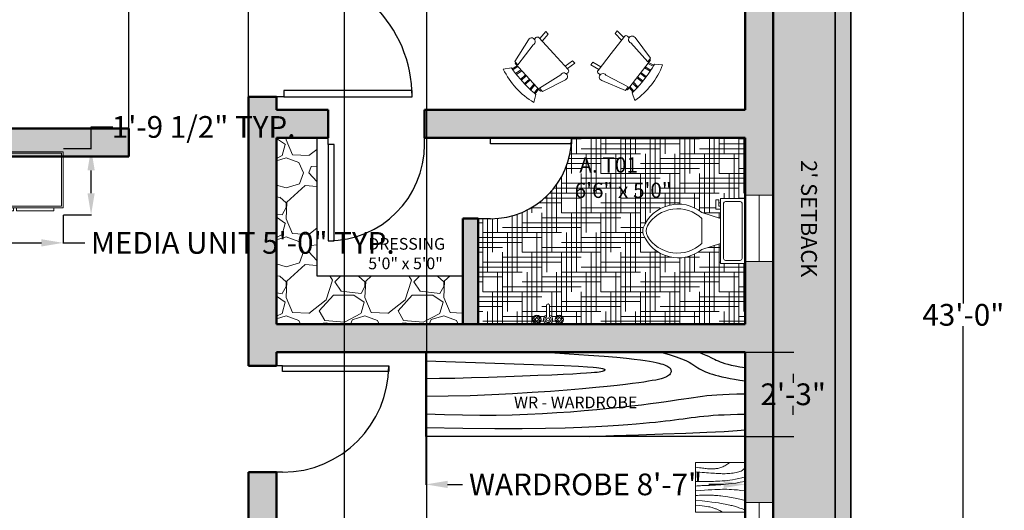
# Model space of a CAD drawing. Units: inches. Extents: x 319 to 870, y 210 to 995.
# Tile 5 of 6: x 524 to 841, y 603 to 761. Entities that reach past the tile are written whole.
import ezdxf

# ---------------------------------------------------------------- set-up
doc = ezdxf.new("R2010")
doc.units = ezdxf.units.IN
doc.header["$MEASUREMENT"] = 0
for name, color, linetype, lineweight in [('A-ANNO-DIMS', 2, 'Continuous', 18), ('A-ANNO-TEXT', 7, 'Continuous', 18), ('A-AREA-IDEN', 7, 'Continuous', 18), ('A-DOOR', 4, 'Continuous', 25), ('A-FLOR-CASE', 7, 'Continuous', 25), ('A-FLOR-CASE-PATT', 252, 'Continuous', 13), ('A-FLOR-FIXT', 9, 'Continuous', 18), ('A-FLOR-PATT', 252, 'Continuous', 13), ('A-FURN', 8, 'Continuous', 18), ('A-GLAZ', 4, 'Continuous', 18), ('A-WALL', 7, 'Continuous', 50), ('A-WALL-PATT', 8, 'Continuous', 13), ('C-PROP', 7, 'Continuous', 35), ('C-PROP-PATT', 8, 'Continuous', 13)]:
    doc.layers.add(name, color=color, linetype=linetype, lineweight=lineweight)
doc.layers.add('C-SITE-PATT', color=126, linetype='Continuous', lineweight=13, true_color=0x1e6f63)
doc.styles.get("Standard").update_dxf_attribs({"font": 'arial.ttf'})
doc.dimstyles.get("Standard").update_dxf_attribs({"dimtxt": 7, "dimasz": 7, "dimexe": 0.18, "dimexo": 0.0625, "dimgap": 0.09, "dimtad": 0, "dimtih": 1, "dimtoh": 1, "dimdec": 0, "dimzin": 0, "dimdsep": 46, "dimlunit": 3, "dimtxsty": 'Standard', "dimcen": 0.09, "dimadec": 0, "dimazin": 0, "dimtfac": 1, "dimtdec": 0, "dimtofl": 0, "dimtmove": 0, "dimatfit": 3, "dimfxl": 1, "dimtolj": 1, "dimtzin": 0, "dimarcsym": 0})

# ---------------------------------------------------------------- blocks, each defined once
blk = doc.blocks.new('Toilet - top')
for p, q in [((9.5, -6), (9.5, -2)), ((-10, -8.5), (-8, -8.5)), ((-10, -9.5), (-10, -8.5)), ((-7, -9.5), (-10, -9.5)), ((-8, -8.5), (-8, -8)), ((-7, -8), (-7, -9.5)), ((-4, -8), (-6, -14)), ((4, -8), (6, -14)), ((4, -14), (-4, -14))]:
    blk.add_line(p, q)
blk.add_lwpolyline([(10.5, -8), (10.5, 0), (-10.5, 0), (-10.5, -8)], close=True)
for points in [[(-9.5, -2), (-9.5, -6)], [(8.5, -1), (-8.5, -1)], [(-8.5, -7), (8.5, -7)]]:
    blk.add_lwpolyline(points)
for centre, radius, start, end in [((-8.62, -1.88), 0.884, 81.8699, 188.1301), ((8.62, -1.88), 0.884, 351.8699, 98.1301), ((-8.62, -6.12), 0.884, 171.8699, 278.1301), ((8.62, -6.12), 0.884, 261.8699, 8.1301), ((3.52, -21.58), 12.17, 141.4691, 247.9714), ((4.2, -21.82), 11.33, 136.3677, 238.9468), ((-3.52, -21.58), 12.17, 292.0284, 38.5307), ((-4.2, -21.82), 11.33, 301.053, 43.6321), ((0, -27.88), 4, 245.7318, 294.2682), ((0, -29), 4, 254.8605, 285.1395)]:
    blk.add_arc(centre, radius, start, end)
blk = doc.blocks.new('Faucet - Bathroom top')
for p, q in [((-4.107, 0.125), (-4.375, 0.125)), ((-3.75, 0.4788), (-3.75, 0.75)), ((-3.5, 0.482), (-3.5, 0.75)), ((-3.1461, 0.125), (-2.875, 0.125)), ((3.143, 0.125), (2.875, 0.125)), ((3.5, 0.4788), (3.5, 0.75)), ((3.75, 0.482), (3.75, 0.75)), ((4.1039, 0.125), (4.375, 0.125)), ((-4.1039, -0.125), (-4.375, -0.125)), ((-3.75, -0.4821), (-3.75, -0.75)), ((-3.5, -0.4789), (-3.5, -0.75)), ((-3.143, -0.125), (-2.875, -0.125)), ((-0.5, -0.8639), (-0.5, -4.5)), ((0.5, -4.5), (0.5, -0.8631)), ((3.1461, -0.125), (2.875, -0.125)), ((3.5, -0.4821), (3.5, -0.75)), ((3.75, -0.4789), (3.75, -0.75)), ((4.107, -0.125), (4.375, -0.125))]:
    blk.add_line(p, q)
for centre, radius in [((-3.625, 0), 1.375), ((-4.625, 0), 0.2795), ((-3.625, 0), 0.5), ((-3.625, 1), 0.2795), ((-2.625, 0), 0.2795), ((0, 0), 0.5), ((3.625, 0), 1.375), ((2.625, 0), 0.2795), ((3.625, 0), 0.5), ((3.625, 1), 0.2795), ((4.625, 0), 0.2795), ((-3.625, -1), 0.2795), ((3.625, -1), 0.2795)]:
    blk.add_circle(centre, radius)
for centre, radius, start, end in [((-3.625, 0), 1, 105.2407, 164.2093), ((-3.625, 0), 1, 16.44125, 74.07887), ((0, 0), 1.5, 289.6514, 250.3603), ((0, 0), 1, 300.3431, 239.7554), ((3.625, 0), 1, 106.12, 164.0884), ((3.625, 0), 1, 16.23422, 73.90469), ((-3.625, 0), 1, 196.2342, 253.9047), ((-3.625, 0), 1, 286.12, 344.0884), ((3.625, 0), 1, 196.4413, 254.0789), ((3.625, 0), 1, 285.2407, 344.2093), ((0, -4.5), 0.5, 180, 0)]:
    blk.add_arc(centre, radius, start, end)
blk = doc.blocks.new('*U14')
for p, q in [((0, 0), (0, -6)), ((-36, 0), (-36, -6))]:
    blk.add_line(p, q)
blk.add_lwpolyline([(0, 0), (0, 36), (-1.75, 36), (-1.75, 0)], close=True)
blk.add_arc((0, 0), 36, 90, 180)
blk = doc.blocks.new('*U15')
for p, q in [((-28, 0), (-28, -6)), ((0, 0), (0, -6))]:
    blk.add_line(p, q)
blk.add_lwpolyline([(0, 0), (0, 28), (-1.75, 28), (-1.75, 0)], close=True)
blk.add_arc((0, 0), 28, 90, 180)
blk = doc.blocks.new('*U16')
for p, q in [((0, 0), (0, -6)), ((32, 0), (32, -6))]:
    blk.add_line(p, q)
blk.add_lwpolyline([(0, 0), (0, 32), (1.75, 32), (1.75, 0)], close=True)
blk.add_arc((0, 0), 32, 0, 90)
blk = doc.blocks.new('Hutch - 19 x 72 in.')
for p, q in [((0, -19), (0, 0)), ((0, 0), (71.999994, 0)), ((71.999994, 0), (71.999994, -19)), ((71.999994, -19), (0, -19))]:
    blk.add_line(p, q)
for points in [[(26.99999, 0), (32.30411, -0.35238), (36.66731, -0.66276), (40.20336, -0.93603), (43.02603, -1.17708), (45.2491, -1.39079), (46.98632, -1.58203), (48.35147, -1.7557), (49.45833, -1.91667), (50.40388, -2.06917), (51.21809, -2.21484), (51.91414, -2.35465), (52.5052, -2.48958), (53.00447, -2.6206), (53.42512, -2.7487), (53.78035, -2.87484), (54.08333, -3), (54.34537, -3.12516), (54.57031, -3.2513), (54.76008, -3.37939), (54.91666, -3.51042), (55.04198, -3.64534), (55.13801, -3.78516), (55.2067, -3.93083), (55.24999, -4.08333), (55.26904, -4.24316), (55.26171, -4.40885), (55.22509, -4.57845), (55.15624, -4.75), (55.05224, -4.92155), (54.91015, -5.09115), (54.72704, -5.25684), (54.49999, -5.41667), (54.22493, -5.56934), (53.89322, -5.71615), (53.49511, -5.85905), (53.02083, -6), (52.4606, -6.14095), (51.80468, -6.28385), (51.04329, -6.43066), (50.16666, -6.58333), (49.16007, -6.74381), (47.98892, -6.91406), (46.61368, -7.09603), (44.99478, -7.29167), (43.09268, -7.50293), (40.86783, -7.73177), (38.28067, -7.98014), (35.29166, -8.25), (31.87654, -8.54053), (28.07226, -8.83984), (23.93107, -9.1333), (19.5052, -9.40625), (14.84692, -9.64404), (10.00846, -9.83203), (5.04207, -9.95557), (0, -10)], [(52.99999, 0), (54.87133, -0.53955), (56.39257, -1.03516), (57.61205, -1.48975), (58.57812, -1.90625), (59.3391, -2.2876), (59.94335, -2.63672), (60.4392, -2.95654), (60.87499, -3.25), (61.29247, -3.52002), (61.70702, -3.76953), (62.12743, -4.00146), (62.56249, -4.21875), (63.02099, -4.42432), (63.51171, -4.62109), (64.04345, -4.81201), (64.62499, -5), (65.26489, -5.1875), (65.9707, -5.375), (66.74975, -5.5625), (67.60937, -5.75), (68.55688, -5.9375), (69.5996, -6.125), (70.744867, -6.3125), (71.999994, -6.5)], [(61.49999, 0), (62.35961, -0.35254), (63.08007, -0.66406), (63.68627, -0.94043), (64.20312, -1.1875), (64.65551, -1.41113), (65.06835, -1.61719), (65.46655, -1.81152), (65.87499, -2), (66.31762, -2.1875), (66.81445, -2.375), (67.38452, -2.5625), (68.04687, -2.75), (68.82055, -2.9375), (69.7246, -3.125), (70.77807, -3.3125), (71.999994, -3.5)], [(0, -2), (11.2006, -2.34123), (19.90169, -2.62044), (26.43969, -2.84595), (31.15103, -3.02604), (34.37214, -3.16903), (36.43945, -3.2832), (37.68936, -3.37687), (38.45833, -3.45833), (39.02937, -3.53459), (39.472, -3.60742), (39.80232, -3.67733), (40.03645, -3.74479), (40.1905, -3.8103), (40.28059, -3.87435), (40.32283, -3.93742), (40.33333, -4), (40.32405, -4.0625), (40.29036, -4.125), (40.22346, -4.1875), (40.11458, -4.25), (39.95491, -4.3125), (39.73567, -4.375), (39.44807, -4.4375), (39.08333, -4.5), (38.62491, -4.56282), (38.02538, -4.6276), (37.22957, -4.69629), (36.18228, -4.77083), (34.82836, -4.85319), (33.11262, -4.94531), (30.97989, -5.04915), (28.37499, -5.16667), (25.27416, -5.29818), (21.77929, -5.4375), (18.02368, -5.57682), (14.14062, -5.70833), (10.26342, -5.82422), (6.52539, -5.91667), (3.05981, -5.97786), (0, -6)], [(71.999994, -9.5), (70.071934, -9.51147), (68.38801, -9.54492), (66.91113, -9.59888), (65.60416, -9.67187), (64.43001, -9.76245), (63.35156, -9.86914), (62.3317, -9.99048), (61.33333, -10.125), (60.32128, -10.27157), (59.26822, -10.43034), (58.14876, -10.60181), (56.93749, -10.78646), (55.60904, -10.98478), (54.13801, -11.19726), (52.49902, -11.4244), (50.66666, -11.66667), (48.62239, -11.92358), (46.37499, -12.19075), (43.9401, -12.46281), (41.33333, -12.73437), (38.57031, -13.00008), (35.66666, -13.25456), (32.63801, -13.49243), (29.49999, -13.70833), (26.26367, -13.89689), (22.92187, -14.05273), (19.46289, -14.17049), (15.875, -14.24479), (12.14648, -14.27026), (8.26562, -14.24154), (4.2207, -14.15324), (0, -14)], [(0, -17), (8.37556, -17.14274), (15.58268, -17.20443), (21.74194, -17.19775), (26.97395, -17.13542), (31.39933, -17.03011), (35.13866, -16.89453), (38.31257, -16.74137), (41.04166, -16.58333), (43.4322, -16.43083), (45.5332, -16.28516), (47.37931, -16.14534), (49.0052, -16.01042), (50.44555, -15.87939), (51.73502, -15.7513), (52.90828, -15.62516), (53.99999, -15.5), (55.04044, -15.37508), (56.04231, -15.25065), (57.01391, -15.1272), (57.96353, -15.00521), (58.89949, -14.88517), (59.83007, -14.76758), (60.76358, -14.65291), (61.70833, -14.54167), (62.6752, -14.43465), (63.68554, -14.33398), (64.76326, -14.24211), (65.93229, -14.16146), (67.21655, -14.09448), (68.63997, -14.04362), (70.226475, -14.01131), (71.999994, -14)], [(36.99999, -19), (42.40038, -18.8125), (47.95312, -18.625), (53.43554, -18.4375), (58.62499, -18.25), (63.29882, -18.0625), (67.23437, -17.875), (70.208978, -17.6875), (71.999994, -17.5)]]:
    blk.add_lwpolyline(points)
blk = doc.blocks.new('Entertainment Center')
for p, q in [((-4, 0), (-5, -1)), ((4, 0), (-4, 0)), ((5, -1), (4, 0)), ((-17, -19), (-17, -1)), ((-17, -1), (43, -1)), ((-16.5, -18.5), (-16.5, -1.5)), ((-16.5, -1.5), (42.5, -1.5)), ((42.5, -1.5), (42.5, -18.5)), ((43, -1), (43, -19)), ((43, -19), (-17, -19)), ((42.5, -18.5), (-16.5, -18.5)), ((-12, -20), (-12, -19)), ((12, -19), (12, -20)), ((15, -20), (15, -19)), ((27, -19), (27, -20)), ((28, -20), (28, -19)), ((40, -19), (40, -20)), ((12, -20), (-12, -20)), ((27, -20), (15, -20)), ((40, -20), (28, -20))]:
    blk.add_line(p, q)
blk.add_arc((0, 40), 61, 259.6111, 280.3889)
blk = doc.blocks.new('Chair - Rocking')
for p, q in [((-8, -4.5), (-10, -1.5)), ((-4.5, -7), (-4.96674, -4.19951)), ((-4, -7), (-4.40532, -4.16272)), ((-1.5, -4.05012), (-1.5, -7)), ((-1, -7), (-1, -4.05012)), ((1, -7), (1, -4.04655)), ((1.5, -4.05012), (1.5, -7)), ((4, -7), (4.40187, -4.18694)), ((4.5, -7), (4.96761, -4.19437)), ((8, -4.5), (10, -1.5)), ((-9, -7.5), (-12, -18.49999)), ((-7, -7.5), (-9, -7.5)), ((-9, -18.49999), (-7, -7.5)), ((-8.23428, -6.99939), (-8.3093, -7.47958)), ((-8.23041, -7), (8.23915, -7)), ((-7.5, -4.5), (-7, -7)), ((-6.5, -7), (-7.02225, -4.43)), ((6.5, -7), (7, -4.4057)), ((7.5, -4.5), (7, -7)), ((7, -7.5), (9, -7.5)), ((9, -18.49999), (7, -7.5)), ((8.31071, -7.48854), (8.23449, -7.00073)), ((9, -7.5), (12, -18.49999)), ((-10.36644, -20.64523), (-10.5, -21.49999)), ((10.5, -21.49999), (10.3575, -20.58798)), ((-9, -22.49999), (-9.5, -26.49999)), ((0, -22.49999), (-9.5, -22.49999)), ((-8, -26.49999), (-7.5, -22.49999)), ((0, -22.49999), (9.5, -22.49999)), ((8, -26.49999), (7.5, -22.49999)), ((9, -22.49999), (9.5, -26.49999)), ((-9.5, -26.49999), (-8, -26.49999)), ((9.5, -26.49999), (8, -26.49999))]:
    blk.add_line(p, q)
for centre, radius, start, end in [((0, -34.08333), 34.08333, 72.93847, 107.0615), ((0, -68.25004), 64.25, 93.92211, 97.15267), ((0, -68.25004), 64.25, 82.84733, 93.92211), ((-10.5, -18.99999), 1.58114, 161.5651, 18.43495), ((-9.5, -21.49999), 1, 180, 270), ((10.5, -18.99999), 1.58114, 161.5651, 18.43495), ((9.5, -21.49999), 1, 270, 0)]:
    blk.add_arc(centre, radius, start, end)
blk = doc.blocks.new('Table - Square Woodgrain 42 x 42 in.')
blk.add_line((0, -42), (42, -42))
for points in [[(0, -4), (1.704, -4.2172), (3.2358, -4.4188), (4.615, -4.604), (5.8615, -4.7721), (6.9951, -4.9224), (8.0357, -5.0541), (9.0031, -5.1667), (9.9171, -5.2594), (10.7951, -5.3316), (11.6445, -5.3836), (12.4702, -5.4157), (13.277, -5.4283), (14.0698, -5.4217), (14.8535, -5.3964), (15.6331, -5.3526), (16.4133, -5.2908), (17.1986, -5.2103), (17.9913, -5.1062), (18.793, -4.9727), (19.6056, -4.8038), (20.4307, -4.5937), (21.2701, -4.3365), (22.1256, -4.0262), (22.9989, -3.6571), (23.888, -3.2272), (24.7756, -2.7516), (25.6408, -2.2491), (26.4624, -1.7387), (27.2195, -1.2395), (27.891, -0.7703), (28.456, -0.3501), (28.8934, 0.002)], [(0, -42), (0, 0), (42, 0), (42, -42)], [(0, -8), (1.8203, -8.1001), (3.6741, -8.2149), (5.5411, -8.3408), (7.4011, -8.4741), (9.2339, -8.6112), (11.0193, -8.7484), (12.7371, -8.8821), (14.3671, -9.0086), (15.8954, -9.1246), (17.3337, -9.2278), (18.6997, -9.3159), (20.0116, -9.387), (21.2871, -9.4389), (22.5442, -9.4696), (23.8008, -9.477), (25.0749, -9.459), (26.3791, -9.4137), (27.7049, -9.3403), (29.0383, -9.2382), (30.3655, -9.1068), (31.6728, -8.9455), (32.9461, -8.7535), (34.1717, -8.5304), (35.3358, -8.2756), (36.4268, -7.9863), (37.443, -7.6521), (38.3849, -7.2603), (39.253, -6.7986), (40.048, -6.2542), (40.7705, -5.6147), (41.421, -4.8674), (42, -4)], [(42, -12), (39.1784, -12.8621), (36.4519, -13.5654), (33.8246, -14.1294), (31.3004, -14.5731), (28.8832, -14.9161), (26.577, -15.1775), (24.3858, -15.3768), (22.3136, -15.5332), (20.3622, -15.6632), (18.5254, -15.7718), (16.7947, -15.8612), (15.1618, -15.9338), (13.6183, -15.9916), (12.1558, -16.0369), (10.7659, -16.0718), (9.4403, -16.0987), (8.1703, -16.1191), (6.9461, -16.1325), (5.7577, -16.1377), (4.595, -16.1335), (3.4479, -16.1188), (2.3064, -16.0924), (1.1604, -16.0532), (0, -16)], [(42, -16), (37.6529, -16.7365), (33.8802, -17.329), (30.6179, -17.7961), (27.8015, -18.1561), (25.3668, -18.4275), (23.2497, -18.6288), (21.3859, -18.7785), (19.7111, -18.8949), (18.1693, -18.9939), (16.7375, -19.0795), (15.401, -19.1534), (14.1449, -19.217), (12.9544, -19.2717), (11.8148, -19.3191), (10.7113, -19.3606), (9.6291, -19.3976), (8.5534, -19.4323), (7.47, -19.4689), (6.3643, -19.5122), (5.222, -19.5672), (4.0288, -19.6386), (2.7703, -19.7313), (1.4321, -19.8501), (0, -20)], [(0, -24), (3.9243, -23.6805), (7.4766, -23.4138), (10.6891, -23.1954), (13.5943, -23.0205), (16.2247, -22.8847), (18.6125, -22.7832), (20.7903, -22.7116), (22.7903, -22.6651), (24.6563, -22.642), (26.4764, -22.6507), (28.35, -22.7024), (30.3766, -22.8084), (32.6555, -22.98), (35.2861, -23.2283), (38.3678, -23.5645), (42, -24)], [(42, -32), (37.392, -31.017), (33.4585, -30.2231), (30.1291, -29.5949), (27.3334, -29.109), (25.0009, -28.742), (23.0612, -28.4707), (21.4439, -28.2716), (20.0786, -28.1215), (18.8998, -28.0002), (17.8609, -27.9014), (16.9206, -27.8219), (16.0371, -27.7588), (15.1691, -27.709), (14.2748, -27.6693), (13.3128, -27.6368), (12.2415, -27.6083), (11.0295, -27.5824), (9.6867, -27.5643), (8.233, -27.5608), (6.6884, -27.5787), (5.0728, -27.6248), (3.4062, -27.7058), (1.7086, -27.8286), (0, -28)], [(0, -32), (5.4026, -32.5358), (9.9494, -33.019), (13.7424, -33.4553), (16.8834, -33.8505), (19.4743, -34.2106), (21.6171, -34.5413), (23.4136, -34.8486), (24.9657, -35.1382), (26.3614, -35.4156), (27.6332, -35.6841), (28.7995, -35.9467), (29.8788, -36.2064), (30.8897, -36.4661), (31.8507, -36.7288), (32.7802, -36.9973), (33.6968, -37.2747), (34.6175, -37.5635), (35.5531, -37.8651), (36.5128, -38.1805), (37.506, -38.5108), (38.5421, -38.8568), (39.6302, -39.2197), (40.7797, -39.6004), (42, -40)], [(0, -36), (3.0098, -36.2857), (5.5354, -36.5643), (7.6368, -36.8359), (9.374, -37.1009), (10.807, -37.3597), (11.9957, -37.6126), (13.0002, -37.8599), (13.8804, -38.102), (14.6874, -38.3393), (15.4365, -38.5729), (16.1338, -38.8041), (16.7858, -39.0341), (17.3987, -39.264), (17.9787, -39.4952), (18.5322, -39.7288), (19.0655, -39.9662), (19.5832, -40.2081), (20.0842, -40.4544), (20.5657, -40.7046), (21.0249, -40.9581), (21.459, -41.2144), (21.8653, -41.4731), (22.2409, -41.7335), (22.5831, -41.9951)]]:
    blk.add_lwpolyline(points)
blk = doc.blocks.new('*U19')
for p, q in [((0, 0), (0, -6)), ((24, 0), (24, -6))]:
    blk.add_line(p, q)
blk.add_lwpolyline([(0, 0), (0, 24), (1.75, 24), (1.75, 0)], close=True)
blk.add_arc((0, 0), 24, 0, 90)
blk = doc.blocks.new('*D29')
at = {"layer": 'A-ANNO-DIMS', "color": 0, "lineweight": -2, "transparency": 16777216}
for p, q in [((477.94, 697.77), (477.94, 688.66)), ((537.94, 697.77), (537.94, 688.66)), ((484.94, 688.84), (530.94, 688.84)), ((537.94, 688.84), (544.94, 688.84))]:
    blk.add_line(p, q, dxfattribs=at)
at = {"layer": 'A-ANNO-DIMS', "color": 0, "transparency": 16777216}
for points in [[(484.94, 690), (484.94, 687.67), (477.94, 688.84)], [(530.94, 690), (530.94, 687.67), (537.94, 688.84)]]:
    blk.add_solid(points, dxfattribs=at)
at = {"layer": 'Defpoints', "color": 0, "transparency": 16777216}
for p in [(477.94, 697.84), (537.94, 697.84), (537.94, 688.84)]:
    blk.add_point(p, dxfattribs=at)
at = {"layer": 'A-ANNO-DIMS', "color": 0, "transparency": 16777216, "insert": (595.82, 688.84), "char_height": 7, "attachment_point": 5}
blk.add_mtext('\\A1;MEDIA UNIT 5\'-0" TYP.', dxfattribs=at)
blk = doc.blocks.new('*D30')
at = {"layer": 'A-ANNO-DIMS', "color": 0, "lineweight": -2, "transparency": 16777216}
for p, q in [((546.94, 719.17), (546.94, 726.17)), ((546.94, 726.17), (553.94, 726.17)), ((538.01, 719.17), (547.12, 719.17)), ((546.94, 704.84), (546.94, 712.17)), ((538.01, 697.84), (547.12, 697.84))]:
    blk.add_line(p, q, dxfattribs=at)
at = {"layer": 'A-ANNO-DIMS', "color": 0, "transparency": 16777216}
for points in [[(545.78, 712.17), (548.11, 712.17), (546.94, 719.17)], [(545.78, 704.84), (548.11, 704.84), (546.94, 697.84)]]:
    blk.add_solid(points, dxfattribs=at)
at = {"layer": 'Defpoints', "color": 0, "transparency": 16777216}
for p in [(537.94, 719.17), (546.94, 719.17), (537.94, 697.84)]:
    blk.add_point(p, dxfattribs=at)
at = {"layer": 'A-ANNO-DIMS', "color": 0, "transparency": 16777216, "insert": (583.19, 726.17), "char_height": 7, "attachment_point": 5}
blk.add_mtext('\\A1;1\'-9 1/2" TYP.', dxfattribs=at)
blk = doc.blocks.new('*D35')
at = {"layer": 'A-ANNO-DIMS', "color": 0, "lineweight": -2, "transparency": 16777216}
for p, q in [((654.78, 626.45), (654.78, 610.9)), ((757.68, 626.45), (757.68, 610.9)), ((661.78, 611.08), (666.54, 611.08)), ((750.68, 611.08), (745.92, 611.08))]:
    blk.add_line(p, q, dxfattribs=at)
at = {"layer": 'A-ANNO-DIMS', "color": 0, "transparency": 16777216}
for points in [[(661.78, 612.24), (661.78, 609.91), (654.78, 611.08)], [(750.68, 612.24), (750.68, 609.91), (757.68, 611.08)]]:
    blk.add_solid(points, dxfattribs=at)
at = {"layer": 'Defpoints', "color": 0, "transparency": 16777216}
for p in [(654.78, 626.51), (757.68, 626.51), (757.68, 611.08)]:
    blk.add_point(p, dxfattribs=at)
at = {"layer": 'A-ANNO-DIMS', "color": 0, "transparency": 16777216, "insert": (706.23, 611.08), "char_height": 7, "attachment_point": 5}
blk.add_mtext('\\A1;WARDROBE 8\'-7"', dxfattribs=at)
blk = doc.blocks.new('*D36')
at = {"layer": 'A-ANNO-DIMS', "color": 0, "lineweight": -2, "transparency": 16777216}
for p, q in [((757.75, 653.67), (773.3, 653.67)), ((773.12, 646.67), (773.12, 643.76)), ((773.12, 633.51), (773.12, 636.42)), ((757.75, 626.51), (773.3, 626.51))]:
    blk.add_line(p, q, dxfattribs=at)
at = {"layer": 'A-ANNO-DIMS', "color": 0, "transparency": 16777216}
for points in [[(771.95, 646.67), (774.29, 646.67), (773.12, 653.67)], [(771.95, 633.51), (774.29, 633.51), (773.12, 626.51)]]:
    blk.add_solid(points, dxfattribs=at)
at = {"layer": 'Defpoints', "color": 0, "transparency": 16777216}
for p in [(757.68, 653.67), (773.12, 653.67), (757.68, 626.51)]:
    blk.add_point(p, dxfattribs=at)
at = {"layer": 'A-ANNO-DIMS', "color": 0, "transparency": 16777216, "insert": (773.12, 640.09), "char_height": 7, "attachment_point": 5}
blk.add_mtext('\\A1;2\'-3"', dxfattribs=at)
blk = doc.blocks.new('*D50')
at = {"layer": 'A-ANNO-DIMS', "color": 0, "lineweight": -2, "transparency": 16777216}
for p, q in [((766.75, 923.67), (828.11, 923.67)), ((827.93, 916.67), (827.93, 669.33)), ((827.93, 414.67), (827.93, 662)), ((757.75, 407.67), (828.11, 407.67))]:
    blk.add_line(p, q, dxfattribs=at)
at = {"layer": 'A-ANNO-DIMS', "color": 0, "transparency": 16777216}
for points in [[(826.77, 916.67), (829.1, 916.67), (827.93, 923.67)], [(826.77, 414.67), (829.1, 414.67), (827.93, 407.67)]]:
    blk.add_solid(points, dxfattribs=at)
at = {"layer": 'Defpoints', "color": 0, "transparency": 16777216}
for p in [(766.68, 923.67), (827.93, 923.67), (757.68, 407.67)]:
    blk.add_point(p, dxfattribs=at)
at = {"layer": 'A-ANNO-DIMS', "color": 0, "transparency": 16777216, "insert": (827.93, 665.67), "char_height": 7, "attachment_point": 5}
blk.add_mtext('\\A1;43\'-0"', dxfattribs=at)
blk = doc.blocks.new('*D55')
at = {"layer": 'A-ANNO-DIMS', "color": 0, "lineweight": -2, "transparency": 16777216}
for p, q in [((628.53, 485.73), (628.53, 985.1)), ((635.53, 984.92), (648.14, 984.92)), ((655.14, 485.73), (655.14, 985.1)), ((655.14, 984.92), (662.14, 984.92))]:
    blk.add_line(p, q, dxfattribs=at)
at = {"layer": 'A-ANNO-DIMS', "color": 0, "transparency": 16777216}
for points in [[(635.53, 986.09), (635.53, 983.75), (628.53, 984.92)], [(648.14, 986.09), (648.14, 983.75), (655.14, 984.92)]]:
    blk.add_solid(points, dxfattribs=at)
at = {"layer": 'Defpoints', "color": 0, "transparency": 16777216}
for p in [(655.14, 984.92), (628.53, 485.67), (655.14, 485.67)]:
    blk.add_point(p, dxfattribs=at)
at = {"layer": 'A-ANNO-DIMS', "color": 0, "transparency": 16777216, "insert": (679.75, 984.92), "char_height": 7, "attachment_point": 5}
blk.add_mtext('\\A1;2\'-2 1/2"', dxfattribs=at)
blk = doc.blocks.new('*D59')
at = {"layer": 'A-ANNO-DIMS', "color": 0, "lineweight": -2, "transparency": 16777216}
for p, q in [((552.06, 984.92), (545.06, 984.92)), ((559.06, 725.73), (559.06, 985.1)), ((597.68, 735.92), (597.68, 985.1)), ((604.68, 984.92), (611.68, 984.92))]:
    blk.add_line(p, q, dxfattribs=at)
at = {"layer": 'A-ANNO-DIMS', "color": 0, "transparency": 16777216}
for points in [[(552.06, 986.09), (552.06, 983.75), (559.06, 984.92)], [(604.68, 986.09), (604.68, 983.75), (597.68, 984.92)]]:
    blk.add_solid(points, dxfattribs=at)
at = {"layer": 'Defpoints', "color": 0, "transparency": 16777216}
for p in [(597.68, 984.92), (597.68, 735.86), (559.06, 725.67)]:
    blk.add_point(p, dxfattribs=at)
at = {"layer": 'A-ANNO-DIMS', "color": 0, "transparency": 16777216, "insert": (578.37, 984.92), "char_height": 7, "attachment_point": 5}
blk.add_mtext('\\A1;3\'-2 1/2"', dxfattribs=at)

msp = doc.modelspace()

# ---------------------------------------------------------------- hatches: boundary and pattern name
at = {"layer": 'A-FLOR-CASE-PATT'}
h = msp.add_hatch(dxfattribs=at)
h.set_pattern_fill('GRAVEL', color=256)
h.set_pattern_definition([(228.01279, (18.288, 25.4), (-203.2, -228.6), [3.4172, -338.30484]), (184.96974, (16.002, 22.86), (304.7999999, 25.4000014), [5.86405, -580.5405]), (132.51045, (10.16, 22.352), (254, -279.4), [4.1348, -409.34723]), (267.27369, (0.254, 16.002), (25.4, 508), [5.34005, -528.66437]), (292.83365, (0, 10.668), (-127, 304.8), [5.23634, -518.39808]), (357.27369, (2.032, 5.842), (-508, 25.4), [5.34005, -528.66437]), (37.69424, (7.366, 5.588), (-330.2, -254), [7.06194, -699.13115]), (72.25533, (12.954, 9.906), (177.8, 558.8), [6.6672, -660.05257]), (121.42957, (14.986, 16.256), (-203.2, 330.2), [5.35813, -530.45546]), (175.23636, (12.192, 20.828), (279.4, -25.4), [6.11713, -299.73937]), (222.39744, (6.096, 21.336), (-304.8, -279.4), [7.91078, -783.16773]), (138.81407, (25.4, 15.748), (-177.8, 152.4), [2.70005, -267.30566]), (171.46923, (23.368, 17.526), (330.2, -50.8), [5.1368, -508.5464]), (225, (18.288, 18.288), (-4e-15, -25.4), [3.5921, -32.3289]), (203.1986, (16.51, 21.336), (127, 50.8), [1.9344, -191.5062]), (291.8014, (14.732, 20.574), (-25.4, 76.2), [2.73566, -134.04753]), (30.96376, (15.748, 18.034), (76.2, 50.8), [4.4432, -143.663]), (161.56505, (19.558, 20.32), (50.8, -25.4), [3.2129, -77.109]), (16.38954, (0, 20.574), (254, 76.2), [4.5009, -445.58827]), (70.34618, (4.318, 21.844), (-101.6, -279.4), [3.776, -373.82216]), (293.1986, (19.558, 25.4), (-50.8, 127), [3.8688, -189.57184]), (343.61046, (21.082, 21.844), (-254, 76.2), [4.5009, -445.58827]), (339.44395, (0, 4.826), (-127, 50.8), [4.34035, -212.67734]), (294.77514, (4.064, 3.302), (-127, 279.4), [3.6367, -360.03593]), (66.8014, (19.812, 0), (50.8, 127), [3.8688, -189.57184]), (17.35402, (21.336, 3.556), (-330.2, -101.6), [4.25783, -421.52376]), (69.44395, (7.366, 0), (-50.8, -127), [2.1702, -214.8475]), (101.30993, (18.288, 0), (-25.4, 101.6), [1.29515, -128.21995]), (165.96376, (18.034, 1.27), (76.2, -25.4), [5.23634, -99.49055]), (186.009, (12.954, 2.54), (254, 25.4), [4.85267, -480.41365]), (303.6901, (15.748, 15.748), (-25.4, 50.8), [3.66324, -87.91776]), (353.15723, (17.78, 12.7), (431.8, -50.8), [6.39557, -633.1601]), (60.9454, (24.13, 11.938), (-101.6, -177.8), [2.6151, -258.8939]), (90, (25.4, 14.224), (-25.4, 25.4), [1.524, -23.876]), (120.25644, (12.446, 3.302), (101.6, -177.8), [3.52867, -349.3394]), (48.01279, (10.668, 6.35), (203.2, 228.6), [6.83443, -334.8876]), (0, (15.24, 11.43), (25.4, 25.4), [6.604, -18.796]), (325.30485, (21.844, 11.43), (254, -177.7999999), [4.0161, -397.59317]), (254.0546, (25.146, 9.144), (-25.4, -101.6), [3.6983, -181.2165]), (207.64598, (24.13, 5.588), (-482.6, -254), [6.02145, -596.12464]), (175.42608, (18.796, 2.794), (-330.2, 25.4), [6.3703, -630.65846])])
h.paths.add_polyline_path([(619.69, 678.22), (619.69, 722.67), (606.68, 722.67), (606.68, 662.67), (666.68, 662.67), (666.68, 678.22)])
at = {"layer": 'A-FLOR-PATT'}
h = msp.add_hatch(dxfattribs=at)
h.set_pattern_fill('HOUND', color=256)
h.set_pattern_definition([(0, (0, 0), (6.35, 1.5875), [25.4, -12.7]), (90, (0, 0), (-1.5875, -6.35), [25.4, -12.7])])
h.paths.add_polyline_path([(749.68, 688.67), (743.69, 686.67, -0.501323), (724.82, 691.62, -0.132891), (724.82, 693.71, -0.501317), (743.68, 698.67), (749.68, 696.67), (749.68, 699.67), (748.18, 699.67), (748.18, 702.67), (749.18, 702.67), (749.18, 700.67), (749.68, 700.67), (749.68, 703.17), (757.68, 703.17), (757.68, 722.67), (701.69, 722.67), (701.69, 720.77), (701.62, 720.77, -0.392996), (675.65, 696.62), (671.68, 696.62), (671.68, 662.67), (690.52, 662.89, -0.791418), (690.4, 663.42), (690.4, 663.68, -0.414214), (690.04, 664.29), (690.04, 664.29), (690.04, 664.02, -1.020482), (691.01, 664.29), (691.27, 664.29, -1.951411), (691.48, 663.89, -0.257992), (690.8, 663.21, -0.455903), (690.52, 662.89), (693.38, 662.88, -0.635614), (693.65, 665.58), (693.65, 668.67, -1), (694.65, 668.67), (694.65, 665.58, -0.842995), (694.15, 662.67), (697.77, 662.89, -0.791418), (697.65, 663.42), (697.65, 663.68, -0.414214), (697.29, 664.29), (697.29, 664.29), (697.29, 664.02, -1.020482), (698.26, 664.29), (698.52, 664.29, -1.951411), (698.73, 663.89, -0.257992), (698.05, 663.21, -0.455903), (697.77, 662.89), (757.68, 662.67), (757.68, 682.17), (749.68, 682.17)])
h.paths.add_polyline_path([(697.5, 665.13, 0.257992), (696.81, 664.45, -0.373717), (697.05, 664.17, -1), (696.49, 664.17, -0.455903), (696.81, 664.45, -0.257992), (697.5, 665.13, -1.072684), (698.05, 665.17, -0.932241)], flags=16)
h.paths.add_polyline_path([(690.25, 665.13, 0.257992), (689.56, 664.45, -0.373717), (689.8, 664.17, -1), (689.24, 664.17, -0.455903), (689.56, 664.45, -0.257992), (690.25, 665.13, -1.072684), (690.8, 665.17, -0.932241)], flags=16)
h.paths.add_polyline_path([(701.24, 700.58), (733.66, 700.58), (733.66, 718.89), (701.24, 718.89)], flags=24)
at = {"layer": 'A-WALL-PATT'}
h = msp.add_hatch(color=256, dxfattribs=at)
h.dxf.hatch_style = 1
h.paths.add_polyline_path([(766.68, 731.67), (766.68, 767.38), (757.68, 767.38), (757.68, 731.67), (654.3, 731.67), (654.3, 722.67), (757.68, 722.67), (757.68, 704.22), (766.68, 704.22)])
h = msp.add_hatch(color=256, dxfattribs=at)
h.dxf.hatch_style = 1
h.paths.add_polyline_path([(405.68, 725.67), (405.68, 753.49), (396.68, 753.49), (396.68, 686.41), (405.68, 686.41), (405.68, 716.67), (537.68, 716.67), (559.06, 716.67), (559.06, 725.67), (528.68, 725.67)])
h = msp.add_hatch(color=256, dxfattribs=at)
h.dxf.hatch_style = 1
h.paths.add_polyline_path([(757.68, 653.67), (757.68, 605.29), (766.68, 605.29), (766.68, 682.86), (757.68, 682.86), (757.68, 662.67), (606.68, 662.67), (606.68, 722.67), (623.34, 722.67), (623.34, 731.67), (606.68, 731.67), (606.68, 735.86), (597.68, 735.86), (597.68, 649.25), (606.68, 649.25), (606.68, 653.67)])
h = msp.add_hatch(color=256, dxfattribs=at)
h.dxf.hatch_style = 1
h.paths.add_polyline_path([(671.68, 696.66), (666.68, 696.66), (666.68, 662.67), (671.68, 662.67)])
h = msp.add_hatch(color=256, dxfattribs=at)
h.dxf.hatch_style = 1
h.paths.add_polyline_path([(606.68, 476.67), (628.53, 476.67), (628.53, 485.67), (606.68, 485.67), (606.68, 614.99), (597.68, 614.99), (597.68, 407.67), (757.68, 407.67), (757.68, 385.48), (766.68, 385.48), (766.68, 431.25), (757.68, 431.25), (757.68, 416.67), (606.68, 416.67)])
at = {"layer": 'C-PROP-PATT'}
h = msp.add_hatch(color=256, dxfattribs=at)
h.dxf.hatch_style = 1
h.paths.add_polyline_path([(757.68, 329.67), (597.68, 329.67), (597.68, 324.67), (791.68, 324.67), (791.68, 948.67), (376.68, 948.67), (376.68, 943.67), (786.68, 943.67), (786.68, 329.67), (766.68, 329.67), (766.68, 354.04), (757.68, 354.04)])
at = {"layer": 'C-SITE-PATT'}
h = msp.add_hatch(color=256, dxfattribs=at)
h.dxf.hatch_style = 1
h.paths.add_polyline_path([(376.68, 515.67), (396.68, 515.67), (396.68, 923.67), (528.68, 923.67), (606.68, 923.67), (766.68, 923.67), (766.68, 329.67), (786.68, 329.67), (786.68, 943.67), (376.68, 943.67)])
h.paths.add_polyline_path([(392.17, 638.98), (392.17, 682.3), (381.61, 682.3), (381.61, 638.98)], flags=24)
h.paths.add_polyline_path([(772.77, 716.95), (772.77, 673.64), (783.33, 673.64), (783.33, 716.95)], flags=24)
h.paths.add_polyline_path([(542.27, 929.56), (581.61, 929.56), (581.61, 939.15), (542.27, 939.15)], flags=24)

# ---------------------------------------------------------------- linework, layer by layer
at = {"layer": 'A-FLOR-CASE'}
for p, q in [((619.69, 722.67), (619.69, 678.22)), ((619.69, 678.22), (666.68, 678.22))]:
    msp.add_line(p, q, dxfattribs=at)
at = {"layer": 'A-GLAZ'}
for p, q in [((757.68, 704.22), (766.68, 704.22)), ((762.18, 704.22), (762.18, 682.86)), ((757.68, 682.86), (766.68, 682.86)), ((757.68, 605.29), (766.68, 605.29)), ((762.18, 605.29), (762.18, 533.56))]:
    msp.add_line(p, q, dxfattribs=at)
at = {"layer": 'A-WALL'}
for p, q in [((766.68, 329.67), (766.68, 923.67)), ((757.68, 914.67), (757.68, 731.67)), ((597.68, 735.86), (606.68, 735.86)), ((597.68, 735.86), (597.68, 649.25)), ((606.68, 735.86), (606.68, 731.67)), ((623.34, 731.67), (606.68, 731.67)), ((623.34, 731.67), (623.34, 722.67)), ((757.68, 731.67), (654.3, 731.67)), ((654.3, 731.67), (654.3, 722.67)), ((766.68, 731.67), (766.68, 329.67)), ((528.68, 725.67), (405.68, 725.67)), ((528.68, 725.67), (559.06, 725.67)), ((559.06, 725.67), (559.06, 716.67)), ((606.68, 722.67), (606.68, 662.67)), ((623.34, 722.67), (606.68, 722.67)), ((757.68, 722.67), (654.3, 722.67)), ((757.68, 722.67), (757.68, 662.67)), ((537.68, 716.67), (405.68, 716.67)), ((559.06, 716.67), (537.68, 716.67)), ((666.68, 696.66), (666.68, 662.67)), ((666.68, 696.66), (671.68, 696.66)), ((671.68, 696.66), (671.68, 662.67)), ((757.68, 662.67), (606.68, 662.67)), ((757.68, 653.67), (606.68, 653.67)), ((606.68, 653.67), (606.68, 649.25)), ((757.68, 653.67), (757.68, 485.67)), ((606.68, 649.25), (597.68, 649.25)), ((597.68, 614.99), (606.68, 614.99)), ((597.68, 614.99), (597.68, 407.67)), ((606.68, 614.99), (606.68, 485.67))]:
    msp.add_line(p, q, dxfattribs=at)
at = {"layer": 'C-PROP'}
for p, q in [((791.68, 324.67), (791.68, 948.67)), ((786.68, 329.67), (786.68, 943.67))]:
    msp.add_line(p, q, dxfattribs=at)

# ---------------------------------------------------------------- block references
at = {"layer": 'A-DOOR'}
for name, p, xscale, yscale, zscale, rotation in [('*U14', (609.07, 735.86), 1.146791488036304, 1.146791488036304, 1.146791488036304, 270), ('*U15', (623.34, 720.52), 1.107835329648236, 1.107835329648236, 1.107835329648236, 180), ('*U19', (675.65, 722.67), 1.085285736553447, 1.085285736553447, 1.085285736553447, 270), ('*U16', (608.6, 649.25), 1.069737115517574, 1.069737115517574, 1.069737115517574, 270)]:
    msp.add_blockref(name, p, dxfattribs=dict(at, xscale=xscale, yscale=yscale, zscale=zscale, rotation=rotation))
at = {"layer": 'A-FLOR-CASE', "xscale": 1.429268313895531, "yscale": 1.429268313895531, "zscale": 1.429268313895531}
msp.add_blockref('Hutch - 19 x 72 in.', (654.78, 653.67), dxfattribs=at)
at = {"layer": 'A-FLOR-FIXT'}
for name, p, rotation in [('Toilet - top', (757.68, 692.67), 270.0000000000009), ('Faucet - Bathroom top', (694.15, 664.17), 180)]:
    msp.add_blockref(name, p, dxfattribs=dict(at, rotation=rotation))
at = {"layer": 'A-FURN'}
for p, xscale, yscale, zscale, rotation in [((683.88, 738.66), 0.7291334553679599, 0.7291334553679599, 0.7291334553679599, 132.650964704195), ((727.45, 739.74), 0.7291334553679598, 0.7291334553679598, 0.7291334553679598, 232.129991157543)]:
    msp.add_blockref('Chair - Rocking', p, dxfattribs=dict(at, xscale=xscale, yscale=yscale, zscale=zscale, rotation=rotation))
msp.add_blockref('Entertainment Center', (494.94, 719.17), dxfattribs=at)
at = {"layer": 'A-FURN', "xscale": 0.3809342412266087, "yscale": 0.3809342412266087, "zscale": 0.3809342412266087}
msp.add_blockref('Table - Square Woodgrain 42 x 42 in.', (741.69, 618.13), dxfattribs=at)

# ---------------------------------------------------------------- texts
at = {"layer": 'A-ANNO-TEXT', "insert": (780.78, 715.46), "char_height": 5.1244, "attachment_point": 1, "rotation": 270}
msp.add_mtext_dynamic_manual_height_columns("2' SETBACK ", width=66.3636, gutter_width=25.62, heights=[0], dxfattribs=at)
at = {"layer": 'A-ANNO-TEXT', "insert": (683.19, 639.36), "char_height": 3.7605, "attachment_point": 1}
msp.add_mtext_dynamic_manual_height_columns('WR - WARDROBE', width=48.7012, gutter_width=18.8, heights=[0], dxfattribs=at)
at = {"layer": 'A-AREA-IDEN', "attachment_point": 1}
for s, width, gutter_width, insert, char_height in [('\\pxi-3,l4,t4; A. T01\\P6\'6" x 5\'0"', 63.5478, 24.53, (697.82, 716.39), 4.9069), ('DRESSING\\P5\'0" x 5\'0"', 48.8305, 18.85, (636.23, 690.41), 3.7705)]:
    msp.add_mtext_dynamic_manual_height_columns(s, width=width, gutter_width=gutter_width, heights=[0], dxfattribs=dict(at, insert=insert, char_height=char_height))

# ---------------------------------------------------------------- dimensions: what is measured, and where the dimension line sits
at = {"layer": 'A-ANNO-DIMS'}
for base, p1, p2, picture, middle in [((597.68, 984.92), (559.06, 725.67), (597.68, 735.86), '*D59', (578.37, 984.92)), ((655.14, 984.92), (628.53, 485.67), (655.14, 485.67), '*D55', (679.75, 984.92))]:
    dim = msp.add_linear_dim(base=base, p1=p1, p2=p2, dimstyle='Standard', override={"dimdec": 1, "dimlfac": 1, "dimrnd": 0, "dimzin": 1, "dimdsep": 46, "dimlunit": 4, "dimfrac": 2}, dxfattribs=at)
    dim.commit()
    dim.dimension.update_dxf_attribs({"geometry": picture, "text_midpoint": middle})
for base, p1, p2, picture, middle in [((827.93, 923.67), (757.68, 407.67), (766.68, 923.67), '*D50', (827.93, 665.67)), ((773.12, 653.67), (757.68, 626.51), (757.68, 653.67), '*D36', (773.12, 640.09))]:
    dim = msp.add_linear_dim(base=base, p1=p1, p2=p2, angle=90, dimstyle='Standard', override={"dimdec": 1, "dimlfac": 1, "dimrnd": 0, "dimzin": 1, "dimdsep": 46, "dimlunit": 4, "dimfrac": 2}, dxfattribs=at)
    dim.commit()
    dim.dimension.update_dxf_attribs({"geometry": picture, "text_midpoint": middle})
dim = msp.add_linear_dim(base=(546.94, 719.17), p1=(537.94, 697.84), p2=(537.94, 719.17), angle=90, text='<> TYP.', dimstyle='Standard', override={"dimdec": 1, "dimlfac": 1, "dimrnd": 0, "dimzin": 1, "dimdsep": 46, "dimlunit": 4, "dimfrac": 2}, dxfattribs=at)
dim.commit()
dim.dimension.update_dxf_attribs({"geometry": '*D30', "text_midpoint": (583.19, 726.17)})
for base, p1, p2, text, picture, middle in [((537.94, 688.84), (477.94, 697.84), (537.94, 697.84), 'MEDIA UNIT <> TYP.', '*D29', (595.82, 688.84)), ((757.68, 611.08), (654.78, 626.51), (757.68, 626.51), 'WARDROBE <>', '*D35', (706.23, 611.08))]:
    dim = msp.add_linear_dim(base=base, p1=p1, p2=p2, text=text, dimstyle='Standard', override={"dimdec": 1, "dimlfac": 1, "dimrnd": 0, "dimzin": 1, "dimdsep": 46, "dimlunit": 4, "dimfrac": 2}, dxfattribs=at)
    dim.commit()
    dim.dimension.update_dxf_attribs({"geometry": picture, "text_midpoint": middle})

doc.saveas('drawing.dxf')
